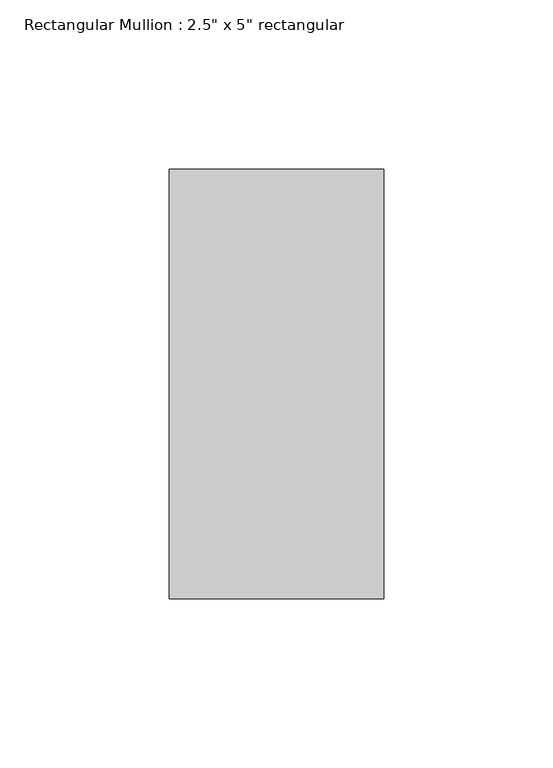
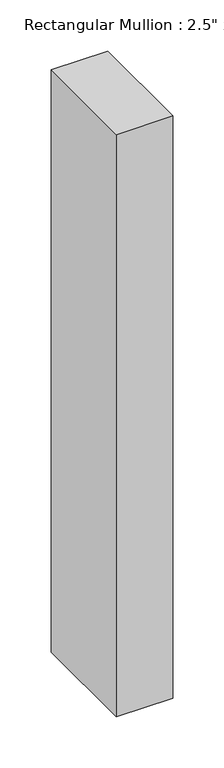
"""IFC4 building model written with IfcOpenShell, lengths in millimetres: member geometry."""

from ifc_helpers import new_model, si_unit, frame, origin, place, context, project, spatial, polyline, outline, extrude, source, transform, mapped, element, save


def member_b59b363a(model_context):
    return source(origin(), model_context, "Body", "SweptSolid", [
        extrude(outline(polyline([(31.75, 63.5), (31.75, -63.5), (-31.75, -63.5), (-31.75, 63.5), (31.75, 63.5)])), frame((0.0, 0.0, -693.4021067), z_axis=(0.0, 0.0, 1.0), x_axis=(1.0, 0.0, 0.0)), (0.0, 0.0, 1.0), 693.4021067),
    ])


if __name__ == "__main__":
    model = new_model("IFC4")
    model_context = context("Model", 3, world=origin())
    ifc_project = project(units=[si_unit("LENGTHUNIT", "METRE", prefix="MILLI")], contexts=[model_context])
    site = spatial("IfcSite", under=ifc_project)
    building = spatial("IfcBuilding", under=site)
    placement = place(None, origin())
    member_shape = member_b59b363a(model_context)
    element("IfcMember", 1, ObjectType="Rectangular Mullion : 2.5\" x 5\" rectangular", at=placement, inside=building, context=model_context, shape_type="MappedRepresentation", body=[
        mapped(member_shape, transform((0.0, 0.0, 0.0), x_axis=(1.0, 0.0, 0.0), y_axis=(0.0, 1.0, 0.0), z_axis=(0.0, 0.0, 1.0))),
    ])
    save(model, "model.ifc")

# Revit data of these elements
# Type "Rectangular Mullion : 2.5\" x 5\" rectangular"
#   built-in parameter 1007304 = 0.416667 (stored number, unit not read)
#   built-in parameter 1007301 = 0.104167 (stored number, unit not read)
#   built-in parameter 1007300 = 0.104167 (stored number, unit not read)
# Element 1 (IfcMember, "Rectangular Mullion : 2.5\" x 5\" rectangular")
#   Materials on its faces: "Aluminum"
# Materials
#   "Aluminum": class "Metal", colour RGB 247 247 247, transparency 0, Description = "Aluminum 6061", Cost = 0
